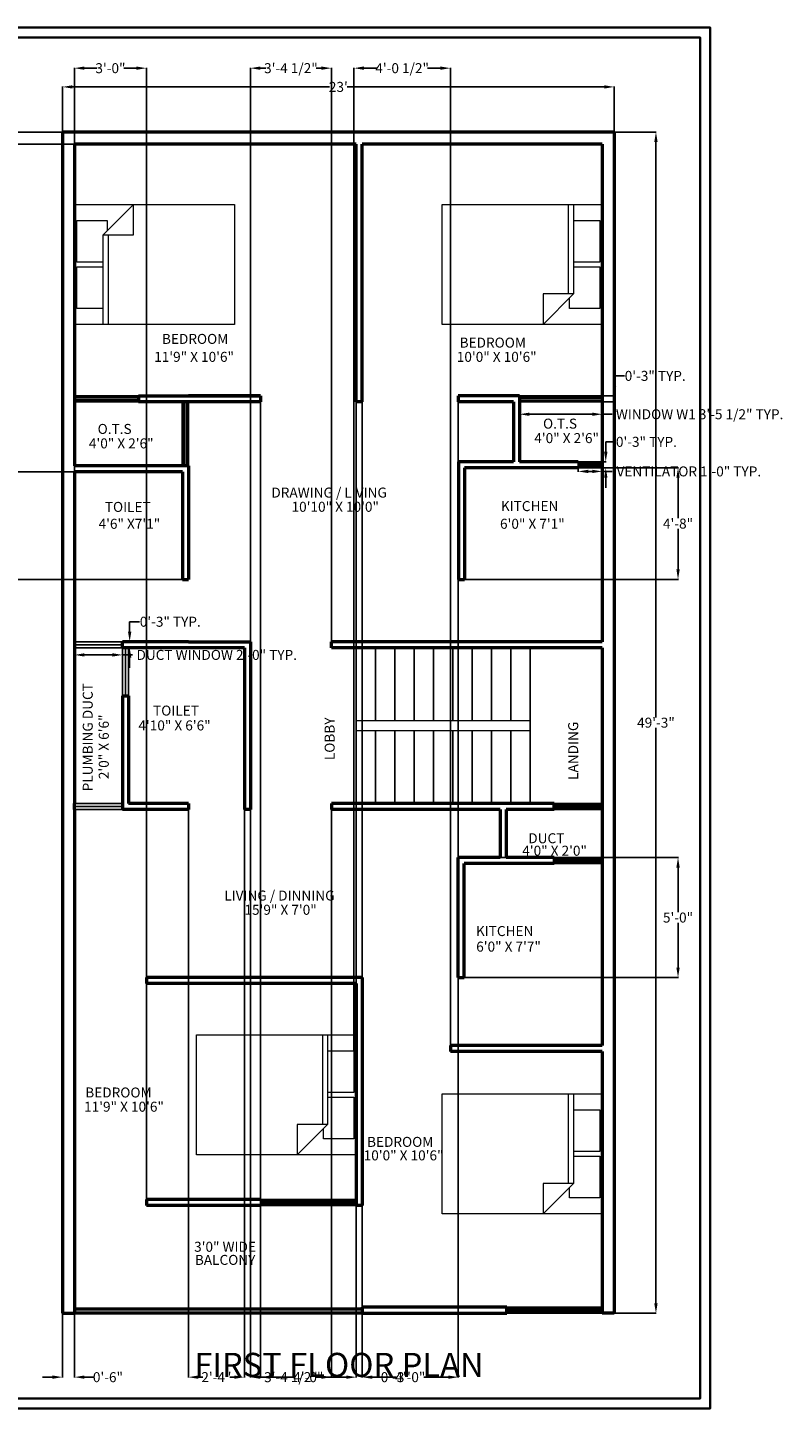
# Model space of a CAD drawing. Units: inches. Extents: x 396 to 1141, y -378 to 313.
# Tile 3 of 3: x 764 to 1141, y -378 to 313. Entities that reach past the tile are written whole.
import ezdxf

# ---------------------------------------------------------------- set-up
doc = ezdxf.new("R2010")
doc.units = ezdxf.units.IN
doc.header["$MEASUREMENT"] = 0
for name, color, linetype, lineweight in [('A-ANNO-DIMS', 2, 'Continuous', 18), ('A-ANNO-TTLB', 7, 'Continuous', 35), ('A-AREA-IDEN', 3, 'Continuous', 25), ('A-FLOR-STRS', 220, 'Continuous', 25), ('A-FURN', 30, 'Continuous', 18), ('A-GLAZ', 4, 'Continuous', 25), ('A-WALL', 7, 'Continuous', 50)]:
    doc.layers.add(name, color=color, linetype=linetype, lineweight=lineweight)
doc.styles.get("Standard").update_dxf_attribs({"font": 'arial.ttf'})
doc.dimstyles.get("Standard").update_dxf_attribs({"dimtxt": 5, "dimasz": 5, "dimexe": 0.18, "dimexo": 0.0625, "dimgap": 0.09, "dimtad": 0, "dimtih": 1, "dimtoh": 1, "dimdec": 1, "dimzin": 0, "dimdsep": 46, "dimlunit": 4, "dimtxsty": 'Standard', "dimcen": 0.09, "dimadec": 0, "dimazin": 0, "dimtfac": 1, "dimtdec": 1, "dimtofl": 0, "dimtmove": 0, "dimatfit": 3, "dimfxl": 1, "dimtolj": 1, "dimtzin": 0, "dimarcsym": 0})

# ---------------------------------------------------------------- blocks, each defined once
blk = doc.blocks.new('Bed - Queen')
for p, q in [((0, -80.00003), (0, 0)), ((0, 0), (59.99999, 0)), ((59.99999, 0), (59.99999, -80.00003)), ((7.99999, -1.2), (28.79998, -1.2)), ((7.99999, -14.4), (7.99999, -1.2)), ((28.79998, -1.2), (28.79998, -14.4)), ((31.19999, -1.2), (51.99999, -1.2)), ((31.19999, -14.4), (31.19999, -1.2)), ((51.99999, -1.2), (51.99999, -16.4)), ((0, -14.4), (44.8, -14.4)), ((44.8, -16.8), (0, -16.8)), ((59.99999, -29.6), (44.8, -14.4)), ((44.8, -14.4), (44.8, -29.6)), ((51.99999, -16.4), (46.79936, -16.4)), ((44.8, -29.6), (59.99999, -29.6)), ((59.99999, -80.00003), (0, -80.00003))]:
    blk.add_line(p, q)
blk = doc.blocks.new('*D11')
at = {"layer": 'A-ANNO-DIMS', "color": 0, "lineweight": -2, "ltscale": 0.3, "transparency": 16777216}
for p, q in [((780.98, 261.02), (780.98, 283.71)), ((785.98, 283.53), (914.61, 283.53)), ((1051.98, 283.53), (923.36, 283.53)), ((1056.98, 261.02), (1056.98, 283.71))]:
    blk.add_line(p, q, dxfattribs=at)
at = {"layer": 'A-ANNO-DIMS', "color": 0, "ltscale": 0.3, "transparency": 16777216}
for points in [[(785.98, 284.36), (785.98, 282.69), (780.98, 283.53)], [(1051.98, 284.36), (1051.98, 282.69), (1056.98, 283.53)]]:
    blk.add_solid(points, dxfattribs=at)
at = {"layer": 'Defpoints', "color": 0, "ltscale": 0.3, "transparency": 16777216}
for p in [(1056.98, 283.53), (780.98, 260.95), (1056.98, 260.95)]:
    blk.add_point(p, dxfattribs=at)
at = {"layer": 'A-ANNO-DIMS', "color": 0, "ltscale": 0.3, "transparency": 16777216, "insert": (918.98, 283.53), "char_height": 5, "attachment_point": 5}
blk.add_mtext("\\A1;23'", dxfattribs=at)
blk = doc.blocks.new('*D12')
at = {"layer": 'A-ANNO-DIMS', "color": 0, "lineweight": -2, "ltscale": 0.3, "transparency": 16777216}
for p, q in [((1057.05, 260.95), (1078.07, 260.95)), ((1077.89, 255.95), (1077.89, -31.9)), ((1077.89, -325.05), (1077.89, -37.19)), ((1057.05, -330.05), (1078.07, -330.05))]:
    blk.add_line(p, q, dxfattribs=at)
at = {"layer": 'A-ANNO-DIMS', "color": 0, "ltscale": 0.3, "transparency": 16777216}
for points in [[(1077.05, 255.95), (1078.72, 255.95), (1077.89, 260.95)], [(1077.05, -325.05), (1078.72, -325.05), (1077.89, -330.05)]]:
    blk.add_solid(points, dxfattribs=at)
at = {"layer": 'Defpoints', "color": 0, "ltscale": 0.3, "transparency": 16777216}
for p in [(1056.98, 260.95), (1056.98, -330.05), (1077.89, -330.05)]:
    blk.add_point(p, dxfattribs=at)
at = {"layer": 'A-ANNO-DIMS', "color": 0, "ltscale": 0.3, "transparency": 16777216, "insert": (1077.89, -34.55), "char_height": 5, "attachment_point": 5}
blk.add_mtext('\\A1;49\'-3"', dxfattribs=at)
blk = doc.blocks.new('WIN-1200')
at = {"ltscale": 0.3}
blk.add_line((664.23, 127.45), (705.61, 127.45), dxfattribs=at)
for points in [[(705.61, 128.95), (664.23, 128.95), (664.23, 125.95), (705.61, 125.95)], [(664.23, 128.38), (705.61, 128.38), (705.61, 126.44), (664.23, 126.44)]]:
    blk.add_lwpolyline(points, close=True, dxfattribs=at)
blk = doc.blocks.new('WIN-VENT-350')
at = {"ltscale": 0.3}
blk.add_line((693.61, 94.45), (705.61, 94.49), dxfattribs=at)
for points in [[(693.61, 95.95), (705.61, 95.95), (705.61, 92.95), (693.61, 92.95)], [(693.61, 95.26), (705.61, 95.26), (705.61, 93.72), (693.61, 93.72)]]:
    blk.add_lwpolyline(points, close=True, dxfattribs=at)
blk = doc.blocks.new('WIN-DUCT-700')
at = {"ltscale": 0.3}
blk.add_line((441.61, 4.45), (465.61, 4.45), dxfattribs=at)
blk.add_lwpolyline([(441.61, 5.95), (465.61, 5.95), (465.61, 2.95), (441.61, 2.95)], close=True, dxfattribs=at)
blk = doc.blocks.new('*D18')
at = {"layer": 'A-ANNO-DIMS', "color": 0, "lineweight": -2, "ltscale": 0.3, "transparency": 16777216}
for p, q in [((786.98, 2.89), (786.98, -0.83)), ((810.98, 2.89), (810.98, -0.83)), ((791.98, -0.65), (805.98, -0.65)), ((810.98, -0.65), (815.98, -0.65))]:
    blk.add_line(p, q, dxfattribs=at)
at = {"layer": 'A-ANNO-DIMS', "color": 0, "ltscale": 0.3, "transparency": 16777216}
for points in [[(791.98, 0.19), (791.98, -1.48), (786.98, -0.65)], [(805.98, 0.19), (805.98, -1.48), (810.98, -0.65)]]:
    blk.add_solid(points, dxfattribs=at)
at = {"layer": 'Defpoints', "color": 0, "ltscale": 0.3, "transparency": 16777216}
for p in [(786.98, 2.95), (810.98, 2.95), (810.98, -0.65)]:
    blk.add_point(p, dxfattribs=at)
at = {"layer": 'A-ANNO-DIMS', "color": 0, "ltscale": 0.3, "transparency": 16777216, "insert": (858.15, -0.65), "char_height": 5, "attachment_point": 5}
blk.add_mtext('\\A1;DUCT WINDOW 2\'-0" TYP.', dxfattribs=at)
blk = doc.blocks.new('*D19')
at = {"layer": 'A-ANNO-DIMS', "color": 0, "lineweight": -2, "ltscale": 0.3, "transparency": 16777216}
for p, q in [((814.58, 10.95), (814.58, 15.95)), ((814.58, 15.95), (819.58, 15.95)), ((811.05, 5.95), (814.76, 5.95)), ((811.05, 2.95), (814.76, 2.95)), ((814.58, -2.05), (814.58, -7.05))]:
    blk.add_line(p, q, dxfattribs=at)
at = {"layer": 'A-ANNO-DIMS', "color": 0, "ltscale": 0.3, "transparency": 16777216}
for points in [[(813.75, 10.95), (815.42, 10.95), (814.58, 5.95)], [(813.75, -2.05), (815.42, -2.05), (814.58, 2.95)]]:
    blk.add_solid(points, dxfattribs=at)
at = {"layer": 'Defpoints', "color": 0, "ltscale": 0.3, "transparency": 16777216}
for p in [(810.98, 5.95), (810.98, 2.95), (814.58, 5.95)]:
    blk.add_point(p, dxfattribs=at)
at = {"layer": 'A-ANNO-DIMS', "color": 0, "ltscale": 0.3, "transparency": 16777216, "insert": (834.91, 15.95), "char_height": 5, "attachment_point": 5}
blk.add_mtext('\\A1;0\'-3" TYP.', dxfattribs=at)
blk = doc.blocks.new('*D20')
at = {"layer": 'A-ANNO-DIMS', "color": 0, "lineweight": -2, "ltscale": 0.3, "transparency": 16777216}
for p, q in [((1009.6, 125.89), (1009.6, 119.57)), ((1050.98, 125.89), (1050.98, 119.57)), ((1014.6, 119.75), (1045.98, 119.75)), ((1050.98, 119.75), (1055.98, 119.75))]:
    blk.add_line(p, q, dxfattribs=at)
at = {"layer": 'A-ANNO-DIMS', "color": 0, "ltscale": 0.3, "transparency": 16777216}
for points in [[(1014.6, 120.58), (1014.6, 118.91), (1009.6, 119.75)], [(1045.98, 120.58), (1045.98, 118.91), (1050.98, 119.75)]]:
    blk.add_solid(points, dxfattribs=at)
at = {"layer": 'Defpoints', "color": 0, "ltscale": 0.3, "transparency": 16777216}
for p in [(1009.6, 125.95), (1050.98, 125.95), (1050.98, 119.75)]:
    blk.add_point(p, dxfattribs=at)
at = {"layer": 'A-ANNO-DIMS', "color": 0, "ltscale": 0.3, "transparency": 16777216, "insert": (1099.74, 119.75), "char_height": 5, "attachment_point": 5}
blk.add_mtext('\\A1;WINDOW W1 3\'-5 1/2" TYP.', dxfattribs=at)
blk = doc.blocks.new('*D21')
at = {"layer": 'A-ANNO-DIMS', "color": 0, "lineweight": -2, "ltscale": 0.3, "transparency": 16777216}
for p, q in [((1057.19, 133.95), (1057.19, 138.95)), ((1057.19, 138.95), (1062.19, 138.95)), ((1051.05, 128.95), (1057.37, 128.95)), ((1051.05, 125.95), (1057.37, 125.95)), ((1057.19, 120.95), (1057.19, 115.95))]:
    blk.add_line(p, q, dxfattribs=at)
at = {"layer": 'A-ANNO-DIMS', "color": 0, "ltscale": 0.3, "transparency": 16777216}
for points in [[(1056.36, 133.95), (1058.03, 133.95), (1057.19, 128.95)], [(1056.36, 120.95), (1058.03, 120.95), (1057.19, 125.95)]]:
    blk.add_solid(points, dxfattribs=at)
at = {"layer": 'Defpoints', "color": 0, "ltscale": 0.3, "transparency": 16777216}
for p in [(1050.98, 128.95), (1050.98, 125.95), (1057.19, 128.95)]:
    blk.add_point(p, dxfattribs=at)
at = {"layer": 'A-ANNO-DIMS', "color": 0, "ltscale": 0.3, "transparency": 16777216, "insert": (1077.52, 138.95), "char_height": 5, "attachment_point": 5}
blk.add_mtext('\\A1;0\'-3" TYP.', dxfattribs=at)
blk = doc.blocks.new('*D22')
at = {"layer": 'A-ANNO-DIMS', "color": 0, "lineweight": -2, "ltscale": 0.3, "transparency": 16777216}
for p, q in [((1038.98, 92.89), (1038.98, 90.97)), ((1043.98, 91.15), (1045.98, 91.15)), ((1050.98, 92.89), (1050.98, 90.97)), ((1050.98, 91.15), (1055.98, 91.15))]:
    blk.add_line(p, q, dxfattribs=at)
at = {"layer": 'A-ANNO-DIMS', "color": 0, "ltscale": 0.3, "transparency": 16777216}
for points in [[(1043.98, 91.99), (1043.98, 90.32), (1038.98, 91.15)], [(1045.98, 91.99), (1045.98, 90.32), (1050.98, 91.15)]]:
    blk.add_solid(points, dxfattribs=at)
at = {"layer": 'Defpoints', "color": 0, "ltscale": 0.3, "transparency": 16777216}
for p in [(1038.98, 92.95), (1050.98, 92.95), (1050.98, 91.15)]:
    blk.add_point(p, dxfattribs=at)
at = {"layer": 'A-ANNO-DIMS', "color": 0, "ltscale": 0.3, "transparency": 16777216, "insert": (1094.34, 91.15), "char_height": 5, "attachment_point": 5}
blk.add_mtext('\\A1;VENTILATOR 1\'-0" TYP.', dxfattribs=at)
blk = doc.blocks.new('*D23')
at = {"layer": 'A-ANNO-DIMS', "color": 0, "lineweight": -2, "ltscale": 0.3, "transparency": 16777216}
for p, q in [((1052.78, 100.95), (1052.78, 105.95)), ((1052.78, 105.95), (1057.78, 105.95)), ((1051.05, 95.95), (1052.96, 95.95)), ((1051.05, 92.95), (1052.96, 92.95)), ((1052.78, 87.95), (1052.78, 82.95))]:
    blk.add_line(p, q, dxfattribs=at)
at = {"layer": 'A-ANNO-DIMS', "color": 0, "ltscale": 0.3, "transparency": 16777216}
for points in [[(1051.95, 100.95), (1053.62, 100.95), (1052.78, 95.95)], [(1051.95, 87.95), (1053.62, 87.95), (1052.78, 92.95)]]:
    blk.add_solid(points, dxfattribs=at)
at = {"layer": 'Defpoints', "color": 0, "ltscale": 0.3, "transparency": 16777216}
for p in [(1050.98, 95.95), (1050.98, 92.95), (1052.78, 95.95)]:
    blk.add_point(p, dxfattribs=at)
at = {"layer": 'A-ANNO-DIMS', "color": 0, "ltscale": 0.3, "transparency": 16777216, "insert": (1073.11, 105.95), "char_height": 5, "attachment_point": 5}
blk.add_mtext('\\A1;0\'-3" TYP.', dxfattribs=at)
blk = doc.blocks.new('*D40')
at = {"layer": 'A-ANNO-DIMS', "color": 0, "lineweight": -2, "ltscale": 0.3, "transparency": 16777216}
for p, q in [((749.03, 265.95), (749.03, 270.95)), ((780.92, 260.95), (748.85, 260.95)), ((786.92, 254.95), (748.85, 254.95)), ((749.03, 249.95), (749.03, 244.95))]:
    blk.add_line(p, q, dxfattribs=at)
at = {"layer": 'A-ANNO-DIMS', "color": 0, "ltscale": 0.3, "transparency": 16777216}
for points in [[(748.2, 265.95), (749.87, 265.95), (749.03, 260.95)], [(748.2, 249.95), (749.87, 249.95), (749.03, 254.95)]]:
    blk.add_solid(points, dxfattribs=at)
at = {"layer": 'Defpoints', "color": 0, "ltscale": 0.3, "transparency": 16777216}
for p in [(780.98, 260.95), (749.03, 254.95), (786.98, 254.95)]:
    blk.add_point(p, dxfattribs=at)
at = {"layer": 'A-ANNO-DIMS', "color": 0, "ltscale": 0.3, "transparency": 16777216, "insert": (749.03, 257.95), "char_height": 5, "attachment_point": 5}
blk.add_mtext('\\A1;0\'-6"', dxfattribs=at)
blk = doc.blocks.new('*D41')
at = {"layer": 'A-ANNO-DIMS', "color": 0, "lineweight": -2, "ltscale": 0.3, "transparency": 16777216}
for p, q in [((780.98, -330.11), (780.98, -362.18)), ((786.98, -328.11), (786.98, -362.18)), ((775.98, -362), (770.98, -362)), ((791.98, -362), (796.98, -362))]:
    blk.add_line(p, q, dxfattribs=at)
at = {"layer": 'A-ANNO-DIMS', "color": 0, "ltscale": 0.3, "transparency": 16777216}
for points in [[(775.98, -361.16), (775.98, -362.83), (780.98, -362)], [(791.98, -361.16), (791.98, -362.83), (786.98, -362)]]:
    blk.add_solid(points, dxfattribs=at)
at = {"layer": 'Defpoints', "color": 0, "ltscale": 0.3, "transparency": 16777216}
for p in [(780.98, -330.05), (786.98, -328.05), (786.98, -362)]:
    blk.add_point(p, dxfattribs=at)
at = {"layer": 'A-ANNO-DIMS', "color": 0, "ltscale": 0.3, "transparency": 16777216, "insert": (803.72, -362), "char_height": 5, "attachment_point": 5}
blk.add_mtext('\\A1;0\'-6"', dxfattribs=at)
blk = doc.blocks.new('*D42')
at = {"layer": 'A-ANNO-DIMS', "color": 0, "lineweight": -2, "ltscale": 0.3, "transparency": 16777216}
for p, q in [((927.98, 125.89), (927.98, -362.18)), ((930.98, 125.89), (930.98, -362.18)), ((922.98, -362), (917.98, -362)), ((935.98, -362), (940.98, -362))]:
    blk.add_line(p, q, dxfattribs=at)
at = {"layer": 'A-ANNO-DIMS', "color": 0, "ltscale": 0.3, "transparency": 16777216}
for points in [[(922.98, -361.16), (922.98, -362.83), (927.98, -362)], [(935.98, -361.16), (935.98, -362.83), (930.98, -362)]]:
    blk.add_solid(points, dxfattribs=at)
at = {"layer": 'Defpoints', "color": 0, "ltscale": 0.3, "transparency": 16777216}
for p in [(927.98, 125.95), (930.98, 125.95), (930.98, -362)]:
    blk.add_point(p, dxfattribs=at)
at = {"layer": 'A-ANNO-DIMS', "color": 0, "ltscale": 0.3, "transparency": 16777216, "insert": (947.72, -362), "char_height": 5, "attachment_point": 5}
blk.add_mtext('\\A1;0\'-3"', dxfattribs=at)
blk = doc.blocks.new('*D43')
at = {"layer": 'A-ANNO-DIMS', "color": 0, "lineweight": -2, "ltscale": 0.3, "transparency": 16777216}
for p, q in [((879.98, 125.89), (879.98, -362.18)), ((927.98, 125.89), (927.98, -362.18)), ((884.98, -362), (897.15, -362)), ((922.98, -362), (910.82, -362))]:
    blk.add_line(p, q, dxfattribs=at)
at = {"layer": 'A-ANNO-DIMS', "color": 0, "ltscale": 0.3, "transparency": 16777216}
for points in [[(884.98, -361.16), (884.98, -362.83), (879.98, -362)], [(922.98, -361.16), (922.98, -362.83), (927.98, -362)]]:
    blk.add_solid(points, dxfattribs=at)
at = {"layer": 'Defpoints', "color": 0, "ltscale": 0.3, "transparency": 16777216}
for p in [(879.98, 125.95), (927.98, 125.95), (927.98, -362)]:
    blk.add_point(p, dxfattribs=at)
at = {"layer": 'A-ANNO-DIMS', "color": 0, "ltscale": 0.3, "transparency": 16777216, "insert": (903.98, -362), "char_height": 5, "attachment_point": 5}
blk.add_mtext('\\A1;4\'-0"', dxfattribs=at)
blk = doc.blocks.new('*D44')
at = {"layer": 'A-ANNO-DIMS', "color": 0, "lineweight": -2, "ltscale": 0.3, "transparency": 16777216}
for p, q in [((930.98, 125.89), (930.98, -362.18)), ((978.98, 125.89), (978.98, -362.18)), ((935.98, -362), (948.15, -362)), ((973.98, -362), (961.82, -362))]:
    blk.add_line(p, q, dxfattribs=at)
at = {"layer": 'A-ANNO-DIMS', "color": 0, "ltscale": 0.3, "transparency": 16777216}
for points in [[(935.98, -361.16), (935.98, -362.83), (930.98, -362)], [(973.98, -361.16), (973.98, -362.83), (978.98, -362)]]:
    blk.add_solid(points, dxfattribs=at)
at = {"layer": 'Defpoints', "color": 0, "ltscale": 0.3, "transparency": 16777216}
for p in [(930.98, 125.95), (978.98, 125.95), (978.98, -362)]:
    blk.add_point(p, dxfattribs=at)
at = {"layer": 'A-ANNO-DIMS', "color": 0, "ltscale": 0.3, "transparency": 16777216, "insert": (954.98, -362), "char_height": 5, "attachment_point": 5}
blk.add_mtext('\\A1;4\'-0"', dxfattribs=at)
blk = doc.blocks.new('*D45')
at = {"layer": 'A-ANNO-DIMS', "color": 0, "lineweight": -2, "ltscale": 0.3, "transparency": 16777216}
for p, q in [((840.92, 90.95), (748.85, 90.95)), ((749.03, 85.95), (749.03, 66.69)), ((749.03, 42.15), (749.03, 61.41)), ((840.92, 37.15), (748.85, 37.15))]:
    blk.add_line(p, q, dxfattribs=at)
at = {"layer": 'A-ANNO-DIMS', "color": 0, "ltscale": 0.3, "transparency": 16777216}
for points in [[(748.2, 85.95), (749.87, 85.95), (749.03, 90.95)], [(748.2, 42.15), (749.87, 42.15), (749.03, 37.15)]]:
    blk.add_solid(points, dxfattribs=at)
at = {"layer": 'Defpoints', "color": 0, "ltscale": 0.3, "transparency": 16777216}
for p in [(840.98, 90.95), (749.03, 37.15), (840.98, 37.15)]:
    blk.add_point(p, dxfattribs=at)
at = {"layer": 'A-ANNO-DIMS', "color": 0, "ltscale": 0.3, "transparency": 16777216, "insert": (749.03, 64.05), "char_height": 5, "attachment_point": 5}
blk.add_mtext('\\A1;4\'-6"', dxfattribs=at)
blk = doc.blocks.new('*D46')
at = {"layer": 'A-ANNO-DIMS', "color": 0, "lineweight": -2, "ltscale": 0.3, "transparency": 16777216}
for p, q in [((982.14, 92.95), (1089.11, 92.95)), ((1088.93, 87.95), (1088.93, 67.69)), ((1088.93, 42.15), (1088.93, 62.41)), ((982.14, 37.15), (1089.11, 37.15))]:
    blk.add_line(p, q, dxfattribs=at)
at = {"layer": 'A-ANNO-DIMS', "color": 0, "ltscale": 0.3, "transparency": 16777216}
for points in [[(1088.1, 87.95), (1089.77, 87.95), (1088.93, 92.95)], [(1088.1, 42.15), (1089.77, 42.15), (1088.93, 37.15)]]:
    blk.add_solid(points, dxfattribs=at)
at = {"layer": 'Defpoints', "color": 0, "ltscale": 0.3, "transparency": 16777216}
for p in [(982.08, 92.95), (982.08, 37.15), (1088.93, 37.15)]:
    blk.add_point(p, dxfattribs=at)
at = {"layer": 'A-ANNO-DIMS', "color": 0, "ltscale": 0.3, "transparency": 16777216, "insert": (1088.93, 65.05), "char_height": 5, "attachment_point": 5}
blk.add_mtext('\\A1;4\'-8"', dxfattribs=at)
blk = doc.blocks.new('*D47')
at = {"layer": 'A-ANNO-DIMS', "color": 0, "lineweight": -2, "ltscale": 0.3, "transparency": 16777216}
for p, q in [((874.98, 6.02), (874.98, 293.08)), ((879.98, 292.9), (882.7, 292.9)), ((910.53, 292.9), (907.82, 292.9)), ((915.53, 6.02), (915.53, 293.08))]:
    blk.add_line(p, q, dxfattribs=at)
at = {"layer": 'A-ANNO-DIMS', "color": 0, "ltscale": 0.3, "transparency": 16777216}
for points in [[(879.98, 293.74), (879.98, 292.07), (874.98, 292.9)], [(910.53, 293.74), (910.53, 292.07), (915.53, 292.9)]]:
    blk.add_solid(points, dxfattribs=at)
at = {"layer": 'Defpoints', "color": 0, "ltscale": 0.3, "transparency": 16777216}
for p in [(915.53, 292.9), (874.98, 5.95), (915.53, 5.95)]:
    blk.add_point(p, dxfattribs=at)
at = {"layer": 'A-ANNO-DIMS', "color": 0, "ltscale": 0.3, "transparency": 16777216, "insert": (895.26, 292.9), "char_height": 5, "attachment_point": 5}
blk.add_mtext('\\A1;3\'-4 1/2"', dxfattribs=at)
blk = doc.blocks.new('*D48')
at = {"layer": 'A-ANNO-DIMS', "color": 0, "lineweight": -2, "ltscale": 0.3, "transparency": 16777216}
for p, q in [((843.98, -78.11), (843.98, -362.18)), ((871.98, -78.11), (871.98, -362.18)), ((848.98, -362), (851.21, -362)), ((866.98, -362), (864.76, -362))]:
    blk.add_line(p, q, dxfattribs=at)
at = {"layer": 'A-ANNO-DIMS', "color": 0, "ltscale": 0.3, "transparency": 16777216}
for points in [[(848.98, -361.16), (848.98, -362.83), (843.98, -362)], [(866.98, -361.16), (866.98, -362.83), (871.98, -362)]]:
    blk.add_solid(points, dxfattribs=at)
at = {"layer": 'Defpoints', "color": 0, "ltscale": 0.3, "transparency": 16777216}
for p in [(843.98, -78.05), (871.98, -78.05), (871.98, -362)]:
    blk.add_point(p, dxfattribs=at)
at = {"layer": 'A-ANNO-DIMS', "color": 0, "ltscale": 0.3, "transparency": 16777216, "insert": (857.98, -362), "char_height": 5, "attachment_point": 5}
blk.add_mtext('\\A1;2\'-4"', dxfattribs=at)
blk = doc.blocks.new('*D49')
at = {"layer": 'A-ANNO-DIMS', "color": 0, "lineweight": -2, "ltscale": 0.3, "transparency": 16777216}
for p, q in [((874.98, -78.11), (874.98, -362.18)), ((915.53, -78.11), (915.53, -362.18)), ((879.98, -362), (882.7, -362)), ((910.53, -362), (907.82, -362))]:
    blk.add_line(p, q, dxfattribs=at)
at = {"layer": 'A-ANNO-DIMS', "color": 0, "ltscale": 0.3, "transparency": 16777216}
for points in [[(879.98, -361.16), (879.98, -362.83), (874.98, -362)], [(910.53, -361.16), (910.53, -362.83), (915.53, -362)]]:
    blk.add_solid(points, dxfattribs=at)
at = {"layer": 'Defpoints', "color": 0, "ltscale": 0.3, "transparency": 16777216}
for p in [(874.98, -78.05), (915.53, -78.05), (915.53, -362)]:
    blk.add_point(p, dxfattribs=at)
at = {"layer": 'A-ANNO-DIMS', "color": 0, "ltscale": 0.3, "transparency": 16777216, "insert": (895.26, -362), "char_height": 5, "attachment_point": 5}
blk.add_mtext('\\A1;3\'-4 1/2"', dxfattribs=at)
blk = doc.blocks.new('*D50')
at = {"layer": 'A-ANNO-DIMS', "color": 0, "lineweight": -2, "ltscale": 0.3, "transparency": 16777216}
for p, q in [((979.05, -102.05), (1089.11, -102.05)), ((1088.93, -107.05), (1088.93, -129.4)), ((1088.93, -157.05), (1088.93, -134.69)), ((979.05, -162.05), (1089.11, -162.05))]:
    blk.add_line(p, q, dxfattribs=at)
at = {"layer": 'A-ANNO-DIMS', "color": 0, "ltscale": 0.3, "transparency": 16777216}
for points in [[(1088.1, -107.05), (1089.77, -107.05), (1088.93, -102.05)], [(1088.1, -157.05), (1089.77, -157.05), (1088.93, -162.05)]]:
    blk.add_solid(points, dxfattribs=at)
at = {"layer": 'Defpoints', "color": 0, "ltscale": 0.3, "transparency": 16777216}
for p in [(978.98, -102.05), (978.98, -162.05), (1088.93, -162.05)]:
    blk.add_point(p, dxfattribs=at)
at = {"layer": 'A-ANNO-DIMS', "color": 0, "ltscale": 0.3, "transparency": 16777216, "insert": (1088.93, -132.05), "char_height": 5, "attachment_point": 5}
blk.add_mtext('\\A1;5\'-0"', dxfattribs=at)
blk = doc.blocks.new('*D51')
at = {"layer": 'A-ANNO-DIMS', "color": 0, "lineweight": -2, "ltscale": 0.3, "transparency": 16777216}
for p, q in [((786.98, -164.98), (786.98, 293.08)), ((791.98, 292.9), (798.24, 292.9)), ((817.95, 292.9), (811.7, 292.9)), ((822.95, -161.98), (822.95, 293.08))]:
    blk.add_line(p, q, dxfattribs=at)
at = {"layer": 'A-ANNO-DIMS', "color": 0, "ltscale": 0.3, "transparency": 16777216}
for points in [[(791.98, 293.74), (791.98, 292.07), (786.98, 292.9)], [(817.95, 293.74), (817.95, 292.07), (822.95, 292.9)]]:
    blk.add_solid(points, dxfattribs=at)
at = {"layer": 'Defpoints', "color": 0, "ltscale": 0.3, "transparency": 16777216}
for p in [(822.95, 292.9), (786.98, -165.05), (822.95, -162.05)]:
    blk.add_point(p, dxfattribs=at)
at = {"layer": 'A-ANNO-DIMS', "color": 0, "ltscale": 0.3, "transparency": 16777216, "insert": (804.97, 292.9), "char_height": 5, "attachment_point": 5}
blk.add_mtext('\\A1;3\'-0"', dxfattribs=at)
blk = doc.blocks.new('*D52')
at = {"layer": 'A-ANNO-DIMS', "color": 0, "lineweight": -2, "ltscale": 0.3, "transparency": 16777216}
for p, q in [((926.75, -198.73), (926.75, 293.08)), ((931.75, 292.9), (938.25, 292.9)), ((970.07, 292.9), (963.57, 292.9)), ((975.07, -196), (975.07, 293.08))]:
    blk.add_line(p, q, dxfattribs=at)
at = {"layer": 'A-ANNO-DIMS', "color": 0, "ltscale": 0.3, "transparency": 16777216}
for points in [[(931.75, 293.74), (931.75, 292.07), (926.75, 292.9)], [(970.07, 293.74), (970.07, 292.07), (975.07, 292.9)]]:
    blk.add_solid(points, dxfattribs=at)
at = {"layer": 'Defpoints', "color": 0, "ltscale": 0.3, "transparency": 16777216}
for p in [(975.07, 292.9), (926.75, -198.79), (975.07, -196.07)]:
    blk.add_point(p, dxfattribs=at)
at = {"layer": 'A-ANNO-DIMS', "color": 0, "ltscale": 0.3, "transparency": 16777216, "insert": (950.91, 292.9), "char_height": 5, "attachment_point": 5}
blk.add_mtext('\\A1;4\'-0 1/2"', dxfattribs=at)
blk = doc.blocks.new('*D53')
at = {"layer": 'A-ANNO-DIMS', "color": 0, "lineweight": -2, "ltscale": 0.3, "transparency": 16777216}
for p, q in [((786.98, -272.98), (786.98, 293.08)), ((791.98, 292.9), (798.24, 292.9)), ((817.95, 292.9), (811.7, 292.9)), ((822.95, -272.98), (822.95, 293.08))]:
    blk.add_line(p, q, dxfattribs=at)
at = {"layer": 'A-ANNO-DIMS', "color": 0, "ltscale": 0.3, "transparency": 16777216}
for points in [[(791.98, 293.74), (791.98, 292.07), (786.98, 292.9)], [(817.95, 293.74), (817.95, 292.07), (822.95, 292.9)]]:
    blk.add_solid(points, dxfattribs=at)
at = {"layer": 'Defpoints', "color": 0, "ltscale": 0.3, "transparency": 16777216}
for p in [(822.95, 292.9), (786.98, -273.05), (822.95, -273.05)]:
    blk.add_point(p, dxfattribs=at)
at = {"layer": 'A-ANNO-DIMS', "color": 0, "ltscale": 0.3, "transparency": 16777216, "insert": (804.97, 292.9), "char_height": 5, "attachment_point": 5}
blk.add_mtext('\\A1;3\'-0"', dxfattribs=at)

msp = doc.modelspace()

# ---------------------------------------------------------------- linework, layer by layer
at = {"layer": 'A-ANNO-TTLB', "ltscale": 0.3}
for points in [[(400.24, 313.19), (1105.01, 313.19), (1105.01, -377.62), (400.24, -377.62)], [(405.24, 308.19), (1100.01, 308.19), (1100.01, -372.62), (405.24, -372.62)]]:
    msp.add_lwpolyline(points, close=True, dxfattribs=at)
at = {"layer": 'A-FLOR-STRS', "ltscale": 0.3}
for p, q in [((927.92, 2.84), (927.92, -33.66)), ((937.59, 2.85), (937.59, -33.65)), ((947.27, 2.87), (947.27, -33.63)), ((956.94, 2.88), (956.94, -33.62)), ((966.62, 2.89), (966.62, -33.61)), ((976.29, 2.9), (976.29, -33.6)), ((985.96, 2.92), (985.96, -33.58)), ((995.64, 2.93), (995.64, -33.57)), ((1005.31, 2.94), (1005.31, -33.56)), ((1014.98, 2.95), (1014.98, -75.05)), ((1014.98, -33.55), (927.92, -33.66)), ((1014.99, -38.55), (927.92, -38.66)), ((927.92, -38.66), (927.92, -75.05)), ((937.59, -38.65), (937.59, -75.15)), ((947.27, -38.63), (947.27, -75.13)), ((956.94, -38.62), (956.94, -75.12)), ((966.62, -38.61), (966.62, -75.11)), ((976.29, -38.6), (976.29, -75.1)), ((985.96, -38.58), (985.96, -75.08)), ((995.64, -38.57), (995.64, -75.07)), ((1005.31, -38.56), (1005.31, -75.06)), ((1014.98, -38.94), (1014.98, -38.91))]:
    msp.add_line(p, q, dxfattribs=at)
at = {"layer": 'A-GLAZ', "ltscale": 0.3}
msp.add_line((812.48, 2.95), (812.48, -21.05), dxfattribs=at)
for points in [[(818.98, 128.95), (818.98, 125.95), (786.98, 125.95), (786.98, 128.95)], [(818.98, 128.31), (818.98, 126.44), (786.98, 126.44), (786.98, 128.31)], [(818.98, 127.9), (818.98, 127.01), (786.98, 127.01), (786.98, 127.9)], [(840.87, 125.95), (843.98, 125.95), (843.98, 93.95), (840.87, 93.95)], [(841.52, 125.95), (843.39, 125.95), (843.39, 93.95), (841.52, 93.95)], [(841.93, 125.95), (842.82, 125.95), (842.82, 93.95), (841.93, 93.95)], [(813.98, 2.95), (813.98, -21.05), (810.98, -21.05), (810.98, 2.95)], [(1026.98, -75.05), (1050.98, -75.05), (1050.98, -78.05), (1026.98, -78.05)], [(1026.98, -75.71), (1050.98, -75.71), (1050.98, -77.4), (1026.98, -77.4)], [(1026.98, -76.14), (1050.98, -76.14), (1050.98, -76.93), (1026.98, -76.93)], [(1026.98, -102.05), (1050.98, -102.05), (1050.98, -105.05), (1026.98, -105.05)], [(1026.98, -102.71), (1050.98, -102.71), (1050.98, -104.4), (1026.98, -104.4)], [(1026.98, -103.14), (1050.98, -103.14), (1050.98, -103.93), (1026.98, -103.93)], [(1053.17, -102.05), (1053.17, -102.05)], [(927.95, -276.05), (880.32, -276.05), (880.32, -273.05), (927.95, -273.05)], [(880.32, -273.58), (927.95, -273.58), (927.95, -275.46), (880.32, -275.46)], [(880.32, -274.11), (927.95, -274.11), (927.95, -274.87), (880.32, -274.87)], [(1050.98, -330.05), (1003.35, -330.05), (1003.35, -327.05), (1050.98, -327.05)], [(1003.35, -327.58), (1050.98, -327.58), (1050.98, -329.46), (1003.35, -329.46)], [(1003.35, -328.11), (1050.98, -328.11), (1050.98, -328.87), (1003.35, -328.87)]]:
    msp.add_lwpolyline(points, close=True, dxfattribs=at)
at = {"layer": 'A-WALL'}
for p, q in [((1056.98, 260.95), (780.98, 260.95)), ((780.98, 260.95), (780.98, -330.05)), ((1056.98, 260.95), (1056.98, -330.05)), ((786.98, 254.95), (786.98, 93.95)), ((927.98, 254.95), (786.98, 254.95)), ((1050.98, 254.95), (930.98, 254.95)), ((1050.98, 254.95), (1050.98, 5.95)), ((879.98, 125.95), (818.98, 125.95)), ((879.98, 128.95), (843.98, 128.95)), ((930.98, 125.95), (927.98, 125.95)), ((1009.6, 128.95), (978.98, 128.95)), ((1006.6, 125.95), (978.98, 125.95)), ((843.98, 93.95), (786.98, 93.95)), ((840.98, 90.95), (786.98, 90.95)), ((786.98, 90.95), (786.98, 5.95)), ((840.98, 90.95), (840.98, 37.15)), ((843.98, 93.95), (843.98, 37.15)), ((1006.6, 95.95), (979.08, 95.95)), ((1038.98, 92.95), (982.08, 92.95)), ((1038.98, 95.95), (1009.6, 95.95)), ((786.98, 5.95), (786.98, 2.95)), ((786.98, 2.95), (786.98, -75.05)), ((843.98, 5.95), (810.98, 5.95)), ((810.98, 2.95), (810.98, 5.95)), ((871.98, 2.95), (810.98, 2.95)), ((1050.98, 5.95), (915.53, 5.95)), ((1050.98, 2.95), (915.53, 2.95)), ((1050.98, 2.95), (1050.98, -196.07)), ((810.98, -21.05), (810.98, -78.05)), ((813.98, -21.05), (813.98, -75.05)), ((786.98, -78.05), (786.98, -75.05)), ((843.98, -75.05), (813.98, -75.05)), ((843.98, -75.05), (843.98, -78.05)), ((1026.98, -75.05), (915.53, -75.05)), ((786.98, -78.05), (786.98, -165.05)), ((843.98, -78.05), (810.98, -78.05)), ((999.98, -78.05), (915.53, -78.05)), ((1026.98, -78.05), (1002.98, -78.05)), ((999.98, -102.05), (978.98, -102.05)), ((1026.98, -102.05), (1002.98, -102.05)), ((1026.98, -105.05), (981.98, -105.05)), ((786.98, -165.05), (786.98, -273.05)), ((927.95, -162.05), (822.95, -162.05)), ((927.95, -165.05), (822.95, -165.05)), ((930.95, -162.05), (927.95, -162.05)), ((927.95, -165.05), (927.95, -273.05)), ((930.95, -162.05), (930.95, -276.05)), ((1050.98, -196.07), (978.98, -196.07)), ((1050.98, -199.07), (978.98, -199.07)), ((1050.98, -199.07), (1050.98, -330.05)), ((786.98, -273.05), (786.98, -330.05)), ((880.32, -273.05), (822.95, -273.05)), ((880.32, -276.05), (822.95, -276.05)), ((927.95, -273.05), (927.95, -276.05)), ((930.95, -276.05), (927.95, -276.05)), ((930.95, -328.05), (786.98, -328.05)), ((930.95, -330.05), (786.98, -330.05)), ((1056.98, -330.05), (1050.98, -330.05))]:
    msp.add_line(p, q, dxfattribs=at)
at = {"layer": 'A-WALL', "ltscale": 0.3}
for p, q in [((927.98, 125.95), (927.98, 254.95)), ((930.98, 125.95), (930.98, 254.95)), ((818.98, 128.95), (879.98, 128.95)), ((818.98, 128.95), (818.98, 125.95)), ((879.98, 128.95), (879.98, 125.95)), ((978.98, 128.95), (978.98, 125.95)), ((1006.6, 125.95), (1006.6, 95.95)), ((1009.6, 128.95), (1009.6, 125.95)), ((1009.6, 125.95), (1009.6, 95.95)), ((979.08, 95.95), (979.08, 92.95)), ((979.08, 92.95), (979.08, 37.15)), ((982.08, 92.95), (982.08, 37.15)), ((840.98, 37.15), (843.98, 37.15)), ((979.08, 37.15), (982.08, 37.15)), ((843.98, 5.95), (871.98, 5.95)), ((871.98, 5.95), (874.98, 5.95)), ((871.98, 2.95), (871.98, -78.05)), ((874.98, 5.95), (874.98, -78.05)), ((915.53, 2.95), (915.53, 5.95)), ((810.98, -21.05), (813.98, -21.05)), ((915.53, -75.05), (915.53, -78.05)), ((1026.98, -78.05), (1026.98, -75.05)), ((1026.98, -75.05), (1026.98, -78.05)), ((874.98, -78.05), (871.98, -78.05)), ((999.98, -78.05), (999.98, -102.05)), ((1002.98, -78.05), (1002.98, -102.05)), ((978.98, -105.05), (978.98, -102.05)), ((1026.98, -102.05), (1026.98, -105.05)), ((978.98, -162.05), (978.98, -105.05)), ((981.98, -162.05), (981.98, -105.05)), ((822.95, -162.05), (823.55, -162.05)), ((822.95, -162.05), (822.95, -165.05)), ((978.98, -162.05), (981.98, -162.05)), ((978.98, -196.07), (975.07, -196.07)), ((975.07, -196.07), (975.07, -199.07)), ((978.98, -199.07), (975.07, -199.07)), ((822.95, -273.05), (822.95, -276.05)), ((880.32, -273.05), (880.32, -276.05)), ((780.98, -330.05), (786.98, -330.05)), ((1003.35, -327.05), (930.95, -327.05)), ((930.95, -327.05), (930.95, -330.05)), ((930.95, -330.05), (1003.35, -330.05)), ((1003.35, -328.11), (1003.35, -327.05)), ((1003.35, -330.05), (1003.35, -328.05))]:
    msp.add_line(p, q, dxfattribs=at)

# ---------------------------------------------------------------- block references
at = {"layer": 'A-FURN', "ltscale": 0.3}
for p, rotation in [((786.98, 164.72), 89.99999999999999), ((1050.98, 224.72), 270), ((927.95, -190.79), 270), ((1050.98, -220.23), 270)]:
    msp.add_blockref('Bed - Queen', p, dxfattribs=dict(at, rotation=rotation))
at = {"layer": 'A-GLAZ'}
for name, p in [('WIN-1200', (345.37, 0)), ('WIN-VENT-350', (345.37, 0)), ('WIN-DUCT-700', (345.37, 0)), ('WIN-DUCT-700', (345.37, -81))]:
    msp.add_blockref(name, p, dxfattribs=at)

# ---------------------------------------------------------------- texts
at = {"layer": 'A-AREA-IDEN', "ltscale": 0.3}
for s, height, p in [('BEDROOM', 5, (830.74, 154.95)), ('BEDROOM', 5, (979.65, 153.09)), ('11\'9" X 10\'6"', 5, (826.85, 145.97)), ('10\'0" X 10\'6"', 5, (978.25, 145.97)), ('O.T.S', 5, (1021.4, 112.56)), ('O.T.S', 5, (798.56, 109.9)), ('4\'0" X 2\'6"', 5, (1017.02, 105.32)), ('4\'0" X 2\'6"', 5, (794.19, 102.67)), ('DRAWING / LIVING', 5, (885.48, 78.06)), ('10\'10" X 10\'0"', 5, (895.58, 70.95)), ('KITCHEN', 5, (1000.3, 71.3)), ('TOILET', 5, (802.17, 70.89)), ('4\'6" X7\'1"', 5, (799.03, 62.45)), ('6\'0" X 7\'1"', 5, (999.87, 62.45)), ('TOILET', 5, (826.29, -31.02)), ('4\'10" X 6\'6"', 5, (818.96, -38.43)), ('DUCT', 5, (1014.01, -94.88)), ('4\'0" X 2\'0"', 5, (1011, -101.12)), ('LIVING / DINNING', 5, (861.91, -123.55)), ('15\'9" X 7\'0"', 5, (872.02, -130.67)), ('KITCHEN', 5, (987.82, -141.31)), ('6\'0" X 7\'7"', 5, (987.96, -149.1)), ('BEDROOM', 5, (792.37, -222.08)), ('11\'9" X 10\'6"', 5, (791.79, -229.19)), ('BEDROOM', 5, (933.34, -246.78)), ('10\'0" X 10\'6"', 5, (931.66, -253.54)), ('3\'0" WIDE', 5, (846.83, -299.27)), ('BALCONY', 5, (847.21, -305.83)), ('FIRST FLOOR PLAN', 12, (846.9, -361.84))]:
    msp.add_text(s, height=height, dxfattribs=at).set_placement(p)
for s, p in [('PLUMBING DUCT', (796.11, -68.93)), ('    2\'0" X 6\'6"', (804.15, -68.93)), ('LOBBY', (917.14, -53.3)), ('LANDING', (1038.98, -63.18))]:
    msp.add_text(s, height=5, rotation=90, dxfattribs=at).set_placement(p)

# ---------------------------------------------------------------- dimensions: what is measured, and where the dimension line sits
at = {"layer": 'A-ANNO-DIMS', "ltscale": 0.3}
for base, p1, p2, picture, middle in [((915.5288, 292.9046), (874.9844, 5.9546), (915.5288, 5.9546), '*D47', (895.2566, 292.9046)), ((975.07, 292.9), (926.75, -198.79), (975.07, -196.07), '*D52', (950.91, 292.9)), ((822.95, 292.9), (786.98, -165.05), (822.95, -162.05), '*D51', (804.97, 292.9)), ((822.95, 292.9), (786.98, -273.05), (822.95, -273.05), '*D53', (804.97, 292.9)), ((927.98, -362), (879.98, 125.95), (927.98, 125.95), '*D43', (903.98, -362)), ((930.98, -362), (927.98, 125.95), (930.98, 125.95), '*D42', (947.72, -362)), ((978.98, -362), (930.98, 125.95), (978.98, 125.95), '*D44', (954.98, -362)), ((871.98, -362), (843.98, -78.05), (871.98, -78.05), '*D48', (857.98, -362)), ((915.5288, -361.9954), (874.9844, -78.0454), (915.5288, -78.0454), '*D49', (895.2566, -361.9954)), ((786.98, -362), (780.98, -330.05), (786.98, -328.05), '*D41', (803.72, -362))]:
    dim = msp.add_linear_dim(base=base, p1=p1, p2=p2, dimstyle='Standard', override={"dimdec": 1, "dimlfac": 1, "dimrnd": 0, "dimzin": 1, "dimdsep": 46, "dimlunit": 4, "dimfrac": 2}, dxfattribs=at)
    dim.commit()
    dim.dimension.update_dxf_attribs({"geometry": picture, "text_midpoint": middle})
dim = msp.add_linear_dim(base=(1056.98, 283.53), p1=(780.98, 260.95), p2=(1056.98, 260.95), dimstyle='Standard', override={"dimclrd": 0, "dimclre": 0, "dimclrt": 0}, dxfattribs=at)
dim.commit()
dim.dimension.update_dxf_attribs({"geometry": '*D11', "text_midpoint": (918.98, 283.53), "dimtype": 160})
for base, p1, p2, override, picture, middle in [((749.03, 254.95), (780.98, 260.95), (786.98, 254.95), {"dimdec": 1, "dimlfac": 1, "dimrnd": 0, "dimzin": 1, "dimdsep": 46, "dimlunit": 4, "dimfrac": 2}, '*D40', (749.03, 257.95)), ((1077.89, -330.05), (1056.98, 260.95), (1056.98, -330.05), {"dimclrd": 0, "dimclre": 0, "dimclrt": 0}, '*D12', (1077.89, -34.55)), ((749.03, 37.15), (840.98, 90.95), (840.98, 37.15), {"dimdec": 1, "dimlfac": 1, "dimrnd": 0, "dimzin": 1, "dimdsep": 46, "dimlunit": 4, "dimfrac": 2}, '*D45', (749.03, 64.05)), ((1088.93, 37.15), (982.08, 92.95), (982.08, 37.15), {"dimdec": 1, "dimlfac": 1, "dimrnd": 0, "dimzin": 1, "dimdsep": 46, "dimlunit": 4, "dimfrac": 2}, '*D46', (1088.93, 65.05)), ((1088.93, -162.05), (978.98, -102.05), (978.98, -162.05), {"dimdec": 1, "dimlfac": 1, "dimrnd": 0, "dimzin": 1, "dimdsep": 46, "dimlunit": 4, "dimfrac": 2}, '*D50', (1088.93, -132.05))]:
    dim = msp.add_linear_dim(base=base, p1=p1, p2=p2, angle=90, dimstyle='Standard', override=override, dxfattribs=at)
    dim.commit()
    dim.dimension.update_dxf_attribs({"geometry": picture, "text_midpoint": middle})
for base, p1, p2, picture, middle in [((1057.19, 128.95), (1050.98, 125.95), (1050.98, 128.95), '*D21', (1077.52, 138.95)), ((1052.78, 95.95), (1050.98, 92.95), (1050.98, 95.95), '*D23', (1073.11, 105.95)), ((814.58, 5.95), (810.98, 2.95), (810.98, 5.95), '*D19', (834.91, 15.95))]:
    dim = msp.add_linear_dim(base=base, p1=p1, p2=p2, angle=90, text='<> TYP.', dimstyle='Standard', override={"dimdec": 1, "dimrnd": 0, "dimzin": 1, "dimlunit": 4, "dimfrac": 2}, dxfattribs=at)
    dim.commit()
    dim.dimension.update_dxf_attribs({"geometry": picture, "text_midpoint": middle})
for base, p1, p2, text, picture, middle in [((1050.98, 119.75), (1009.6, 125.95), (1050.98, 125.95), 'WINDOW W1 <> TYP.', '*D20', (1099.74, 119.75)), ((1050.98, 91.15), (1038.98, 92.95), (1050.98, 92.95), 'VENTILATOR <> TYP.', '*D22', (1094.34, 91.15)), ((810.98, -0.65), (786.98, 2.95), (810.98, 2.95), 'DUCT WINDOW <> TYP.', '*D18', (858.15, -0.65))]:
    dim = msp.add_linear_dim(base=base, p1=p1, p2=p2, text=text, dimstyle='Standard', override={"dimdec": 1, "dimrnd": 0, "dimzin": 1, "dimlunit": 4, "dimfrac": 2}, dxfattribs=at)
    dim.commit()
    dim.dimension.update_dxf_attribs({"geometry": picture, "text_midpoint": middle})

doc.saveas('drawing.dxf')
